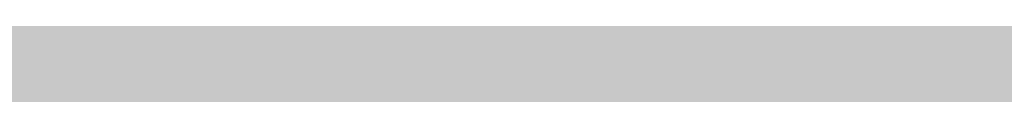
# Model space of a CAD drawing. Units: inches. Extents: x 2083 to 3317, y 1141 to 2115.
# Tile 153 of 256: x 3126.946713 to 3126.955939, y 1263.261932 to 1263.262504. Entities that reach past the tile are written whole.
import ezdxf

# ---------------------------------------------------------------- set-up
doc = ezdxf.new("R2010")
doc.units = ezdxf.units.IN
doc.layers.add('A-ANNO-DIMS', color=2, linetype='Continuous', lineweight=18)
doc.layers.add('A-WALL-PATT', color=251, linetype='Continuous', lineweight=13, true_color=0x636466)
doc.styles.get("Standard").update_dxf_attribs({"font": 'arial.ttf'})
doc.dimstyles.new('ISO-25', dxfattribs={"dimtxt": 12, "dimasz": 12, "dimexe": 1.25, "dimexo": 0.625, "dimtad": 1, "dimlunit": 3, "dimtxsty": 'Standard', "dimcen": 2.5, "dimadec": 0, "dimazin": 0, "dimtfac": 1, "dimtmove": 0, "dimatfit": 3, "dimfxl": 1, "dimarcsym": 0})

# ---------------------------------------------------------------- blocks, each defined once
blk = doc.blocks.new('*D26')
at = {"layer": 'A-ANNO-DIMS', "color": 0, "lineweight": -2, "transparency": 16777216}
for p, q in [((3088.985844, 1274.915092), (3088.985844, 1270.9519631)), ((3111.2400366, 1274.915092), (3111.2400366, 1270.9519631)), ((3076.985844, 1272.2019631), (2840.262447, 1272.2019631)), ((3111.2400366, 1272.2019631), (3088.985844, 1272.2019631)), ((3123.2400366, 1272.2019631), (3135.2400366, 1272.2019631))]:
    blk.add_line(p, q, dxfattribs=at)
at = {"layer": 'A-ANNO-DIMS', "color": 0, "transparency": 16777216}
for points in [[(3076.985844, 1274.2019631), (3076.985844, 1270.2019631), (3088.985844, 1272.2019631)], [(3123.2400366, 1274.2019631), (3123.2400366, 1270.2019631), (3111.2400366, 1272.2019631)]]:
    blk.add_solid(points, dxfattribs=at)
at = {"layer": 'Defpoints', "color": 0, "transparency": 16777216}
for p in [(3088.985844, 1275.540092), (3111.2400366, 1275.540092), (3088.985844, 1272.2019631)]:
    blk.add_point(p, dxfattribs=at)
at = {"layer": 'A-ANNO-DIMS', "color": 0, "transparency": 16777216, "insert": (2952.6241455, 1279.0316016), "char_height": 12, "attachment_point": 5}
blk.add_mtext('NIGHTSTAND 1\'-10 1/2" TYP.', dxfattribs=at)

msp = doc.modelspace()

# ---------------------------------------------------------------- hatches: boundary and pattern name
at = {"layer": 'A-WALL-PATT'}
h = msp.add_hatch(color=256, dxfattribs=at)
h.dxf.hatch_style = 1
h.paths.add_polyline_path([(3126.9597832, 2020.7613601), (2748.9597832, 2020.7613601), (2604.9597832, 2020.7613601), (2226.9597832, 2020.7613601), (2226.9597832, 1702.7613601), (2466.9597832, 1702.7613601), (2466.9597832, 1582.7613601), (2418.9597832, 1582.7613601), (2418.9597832, 1477.7613601), (2226.9597832, 1477.7613601), (2226.9597832, 1263.2613601), (2544.9597832, 1263.2613601), (2544.9597832, 1411.7613601), (2604.9597832, 1411.7613601), (2685.9597832, 1411.7613601), (2685.9597832, 1420.7613601), (2604.9597832, 1420.7613601), (2604.9597832, 1573.7613601), (2604.9597832, 1702.7613601), (2604.9597832, 2011.7613601), (2748.9597832, 2011.7613601), (2748.9597832, 1702.7613601), (2862.9597832, 1702.7613601), (2862.9597832, 1621.7613601), (2871.9597832, 1621.7613601), (2871.9597832, 1702.7613601), (2883.9597832, 1702.7613601), (2883.9597832, 1706.9394595, -0.026459), (2883.9597832, 1711.7613601), (2757.9597832, 1711.7613601), (2757.9597832, 1807.7613601), (2787.9597832, 1807.7613601), (2787.9597832, 1812.2613601), (2757.9597832, 1812.2613601), (2757.9597832, 2011.7613601), (2877.9597832, 2011.7613601), (2877.9597832, 1812.2613601), (2847.9597832, 1812.2613601), (2847.9597832, 1807.7613601), (2889.8357425, 1807.7613601), (2889.8357425, 1812.2613601), (2882.4597832, 1812.2613601), (2882.4597832, 2011.7613601), (3117.9597832, 2011.7613601), (3117.9597832, 1812.2613601), (2937.8357425, 1812.2613601), (2937.8357425, 1807.7613601), (2995.7097832, 1807.7613601), (2995.7097832, 1796.1176655), (3000.2097832, 1796.1176655), (3000.2097832, 1807.7613601), (3117.9597832, 1807.7613601), (3117.9597832, 1711.7613601), (3000.2097832, 1711.7613601), (3000.2097832, 1760.1176655), (2998.5727047, 1760.1176655, -0.020711), (2995.7097832, 1760.1176655), (2995.7097832, 1711.7613601), (2931.9597832, 1711.7613601), (2931.9597832, 1702.7613601), (3126.9597832, 1702.7613601)])
h.paths.add_polyline_path([(2471.4597832, 2011.7613601), (2471.4597832, 1810.0113601), (2462.7169357, 1810.0113601), (2462.7169357, 1805.5113601), (2505.9597832, 1805.5113601), (2505.9597832, 1810.0113601), (2475.9597832, 1810.0113601), (2475.9597832, 2011.7613601), (2595.9597832, 2011.7613601), (2595.9597832, 1810.0113601), (2565.9597832, 1810.0113601), (2565.9597832, 1805.5113601), (2595.9597832, 1805.5113601), (2595.9597832, 1711.7613601), (2235.9597832, 1711.7613601), (2235.9597832, 1805.5113601), (2353.7097832, 1805.5113601), (2353.7097832, 1796.0541624), (2358.2097832, 1796.0541624), (2358.2097832, 1805.5113601), (2414.7169357, 1805.5113601), (2414.7169357, 1810.0113601), (2235.9597832, 1810.0113601), (2235.9597832, 2011.7613601)], flags=16)
h.paths.add_polyline_path([(2270.2047343, 1994.6100082), (2270.2047343, 1970.6100082), (2246.2047343, 1970.6100082), (2246.2047343, 1994.6100082)], flags=0)
edge = h.paths.add_edge_path(flags=0)
edge.add_ellipse((2332.027391, 1899.7981761), major_axis=(-3.0429938, 3.0429938), ratio=0.16825245, start_angle=-161.3321656, end_angle=-156.3071136, ccw=False)
edge.add_ellipse((2333.0820373, 1898.7435297), major_axis=(-1.0546463, 1.0546463), ratio=0.453532097, start_angle=-123.371019, end_angle=-94.1591066)
edge = h.paths.add_edge_path(flags=0)
edge.add_ellipse((2332.027391, 1968.8762897), major_axis=(3.0429938, 3.0429938), ratio=0.16825245, start_angle=18.6678344, end_angle=23.6928864)
edge.add_spline(control_points=[(2332.9255964, 1970.6911045), (2332.2267681, 1970.3360997), (2330.8937087, 1969.6589054), (2328.4130803, 1970.9321376), (2327.2039345, 1967.7487119), (2324.7095965, 1969.9555886), (2322.5328223, 1967.012354), (2320.0128462, 1971.2958124), (2317.6803077, 1968.1578449), (2316.0405263, 1967.1020468), (2315.4269045, 1966.8096022)], knot_values=[0, 0, 0, 0, 2.267059, 4.324559, 6.685584, 8.878641, 11.121502, 14.300359, 17.755284, 19.732645, 19.732645, 19.732645, 19.732645], degree=3, periodic=0)
edge.add_ellipse((2332.027391, 1968.8762897), major_axis=(3.0429938, 3.0429938), ratio=0.16825245, start_angle=18.6678344, end_angle=23.6928864, ccw=False)
edge.add_ellipse((2333.0820373, 1969.930936), major_axis=(1.0546463, 1.0546463), ratio=0.453532097, start_angle=56.628981, end_angle=85.8408934, ccw=False)
edge = h.paths.add_edge_path(flags=0)
edge.add_spline(control_points=[(2296.4282874, 1967.9879081), (2293.6278045, 1965.3363137), (2287.7036238, 1959.727094), (2299.7438601, 1949.9956993), (2294.5325909, 1935.6685275), (2290.5732281, 1920.6035119), (2293.3941244, 1909.9736911), (2296.1854073, 1904.9665431)], knot_values=[0.099185, 0.099185, 0.099185, 0.099185, 0.345301, 0.619822, 0.982653, 1.386093, 1.810555, 1.810555, 1.810555, 1.810555], degree=3, periodic=0)
edge.add_spline(control_points=[(2296.1854073, 1904.9665431), (2297.3835817, 1902.6193002), (2298.0009694, 1901.9493116), (2298.5529698, 1901.4681549)], knot_values=[0.006246, 0.006246, 0.006246, 0.006246, 0.055476, 0.055476, 0.055476, 0.055476], degree=3, periodic=0)
edge.add_spline(control_points=[(2298.5529698, 1901.4681549), (2297.2586121, 1900.9232238), (2295.2252939, 1900.2321257), (2293.0602287, 1900.6142053), (2292.1014227, 1900.788415), (2292.0895776, 1900.790568)], knot_values=[0.312835, 0.312835, 0.312835, 0.312835, 0.40178, 0.474987, 0.475903, 0.475903, 0.475903, 0.475903], degree=3, periodic=0)
edge.add_arc((2292.7936464, 1904.6641088), 3.9370079, 215.4208969, 259.6981795, ccw=False)
edge.add_spline(control_points=[(2289.5853139, 1902.3823039), (2289.4766524, 1902.5350874), (2289.3684805, 1902.6880353), (2289.2608648, 1902.8411699)], knot_values=[0.102872, 0.102872, 0.102872, 0.102872, 0.116896, 0.116896, 0.116896, 0.116896], degree=3, periodic=0)
edge.add_spline(control_points=[(2289.2608648, 1902.8411699), (2288.6866042, 1902.5501922), (2287.6400477, 1902.0199025), (2285.8813368, 1901.8739536), (2283.8529717, 1901.5043521), (2281.7199871, 1899.7105375), (2278.4669913, 1899.492942), (2276.1571361, 1901.8832022), (2272.2589526, 1899.8040711), (2267.7776054, 1901.8431828), (2262.2438819, 1900.1840326), (2257.414927, 1901.7820606), (2254.318374, 1900.7261196), (2253.1782849, 1900.3373431)], knot_values=[0, 0, 0, 0, 1.907977, 3.477176, 5.261074, 7.972851, 11.680248, 13.717921, 16.939592, 22.789562, 27.502503, 33.595215, 37.145618, 37.145618, 37.145618, 37.145618], degree=3, periodic=0)
edge.add_line((2253.1782849, 1900.3373431), (2250.2442397, 1902.8411699))
edge.add_line((2250.2442397, 1902.8411699), (2250.2442397, 1965.8332959))
edge.add_line((2250.2442397, 1965.8332959), (2253.1782849, 1968.3371226))
edge.add_spline(control_points=[(2253.1782849, 1968.3371226), (2254.318374, 1967.9483462), (2257.414927, 1966.8924051), (2262.2438819, 1968.4904332), (2267.7776054, 1966.8312829), (2271.5267301, 1968.5372172), (2273.8759143, 1967.8282895), (2274.2067012, 1967.7276424)], knot_values=[0, 0, 0, 0, 0.09018, 0.244935, 0.364644, 0.513233, 0.537855, 0.537855, 0.537855, 0.537855], degree=3, periodic=0)
edge.add_arc((2274.3528869, 1963.7933495), 3.9370079, 72.0511336, 92.1279492, ccw=False)
edge.add_arc((2281.2969331, 1985.2300027), 18.5962982, 252.05113361, 288.56572166)
edge.add_arc((2292.3167172, 1956.0288805), 12.6460805, 71.02678788, 113.77821843, ccw=False)
edge = h.paths.add_edge_path(flags=0)
edge.add_spline(control_points=[(2274.8994147, 1951.8561946), (2275.066156, 1951.6165924), (2275.2326866, 1951.3765878), (2275.3979871, 1951.1358545)], knot_values=[1.409916, 1.409916, 1.409916, 1.409916, 1.43159, 1.43159, 1.43159, 1.43159], degree=3, periodic=0)
edge.add_spline(control_points=[(2275.3979871, 1951.1358545), (2275.7921055, 1950.5618854), (2276.1792311, 1949.9837745), (2276.5455462, 1949.3971029)], knot_values=[1.358238, 1.358238, 1.358238, 1.358238, 1.409916, 1.409916, 1.409916, 1.409916], degree=3, periodic=0)
edge.add_line((2276.5455462, 1949.3971029), (2277.437289, 1947.8621847))
edge.add_spline(control_points=[(2277.437289, 1947.8621847), (2276.3038341, 1945.6731147), (2274.6396979, 1942.4268817), (2274.631615, 1938.0938998), (2272.7991237, 1930.8515498), (2274.3564261, 1943.8970461), (2275.9476814, 1947.9233558), (2276.5455462, 1949.3971029)], knot_values=[0.005632, 0.005632, 0.005632, 0.005632, 0.186014, 0.266002, 0.357087, 0.59639, 0.739732, 0.739732, 0.739732, 0.739732], degree=3, periodic=0)
edge.add_spline(control_points=[(2276.5455462, 1949.3971029), (2276.1792311, 1949.9837745), (2275.7921055, 1950.5618854), (2275.3979871, 1951.1358545)], knot_values=[1.358238, 1.358238, 1.358238, 1.358238, 1.409916, 1.409916, 1.409916, 1.409916], degree=3, periodic=0)
edge.add_spline(control_points=[(2275.3979871, 1951.1358545), (2274.9425002, 1950.0804523), (2274.2077604, 1948.0252718), (2273.9346018, 1944.8514774), (2272.4685341, 1937.6274891), (2273.4662155, 1945.6964663), (2274.7006154, 1951.0594725), (2274.8994147, 1951.8561946)], knot_values=[0.104364, 0.104364, 0.104364, 0.104364, 0.189636, 0.269624, 0.36071, 0.600013, 0.644622, 0.644622, 0.644622, 0.644622], degree=3, periodic=0)
h.paths.add_polyline_path([(2269.1675139, 1963.1275729, -0.357527), (2268.170633, 1960.9763695, -0.092561), (2268.170633, 1939.4363249, -0.357527), (2269.1675139, 1937.2851215, -0.357527), (2267.0163105, 1938.2820024, -0.164785), (2254.6855813, 1938.2820024, -0.357527), (2252.5343779, 1937.2851215, -0.357527), (2253.5312587, 1939.4363249, -0.092561), (2253.5312587, 1960.9763695, -0.357527), (2252.5343779, 1963.1275729, -0.357527), (2254.6855813, 1962.130692, -0.164785), (2267.0163105, 1962.130692, -0.357527)], flags=0)
h.paths.add_polyline_path([(2248.8740679, 1967.8017998), (2248.8740679, 1957.0277095), (2249.4577833, 1957.0277095), (2249.4577833, 1911.6467562), (2248.8740679, 1911.6467562), (2248.8740679, 1900.8726659), (2246.5118632, 1900.8726659, 0.197327), (2244.1496584, 1902.4568734), (2244.1496584, 1966.2175923, 0.197327), (2246.5118632, 1967.8017998)], flags=0)
h.paths.add_polyline_path([(2269.1675139, 1931.3893442, -0.357527), (2268.170633, 1929.2381408, -0.092561), (2268.170633, 1907.6980962, -0.357527), (2269.1675139, 1905.5468928, -0.357527), (2267.0163105, 1906.5437737, -0.164785), (2254.6855813, 1906.5437737, -0.357527), (2252.5343779, 1905.5468928, -0.357527), (2253.5312587, 1907.6980962, -0.092561), (2253.5312587, 1929.2381408, -0.357527), (2252.5343779, 1931.3893442, -0.357527), (2254.6855813, 1930.3924634, -0.164785), (2267.0163105, 1930.3924634, -0.357527)], flags=0)
edge = h.paths.add_edge_path(flags=0)
edge.add_spline(control_points=[(2276.1968578, 1906.7237016), (2276.1681442, 1909.0289278), (2276.1140492, 1913.371852), (2270.5984171, 1924.9249783), (2273.9051746, 1919.0127787), (2275.9217115, 1916.2620626), (2275.4745699, 1912.4021495), (2277.2578735, 1910.3806206), (2276.6960436, 1908.2250358), (2276.6462176, 1906.8130226), (2276.6178249, 1906.0084068)], knot_values=[0, 0, 0, 0, 8.61026, 16.221274, 18.843057, 23.804898, 27.440828, 29.356102, 31.203478, 33.650687, 33.650687, 33.650687, 33.650687], degree=3, periodic=0)
edge.add_spline(control_points=[(2276.6178249, 1906.0084068), (2276.6233131, 1905.6241436), (2276.4977381, 1904.6286608), (2275.4417789, 1903.8547251), (2274.9373144, 1903.0804497), (2274.8590804, 1902.8411699)], knot_values=[0.156488, 0.156488, 0.156488, 0.156488, 0.184398, 0.231376, 0.250598, 0.250598, 0.250598, 0.250598], degree=3, periodic=0)
edge.add_line((2274.8590804, 1902.8411699), (2276.50598, 1902.8411699))
edge.add_spline(control_points=[(2276.50598, 1902.8411699), (2276.7883084, 1903.0849395), (2277.6650711, 1904.1251958), (2278.2495378, 1904.340738), (2277.6538719, 1908.5273866), (2278.15567, 1906.2278078), (2278.100464, 1905.2859484), (2278.8466748, 1904.0690054), (2277.8567853, 1903.4149482), (2277.8741909, 1902.9910497), (2277.9035616, 1902.8411699)], knot_values=[0.059574, 0.059574, 0.059574, 0.059574, 0.080753, 0.103741, 0.16972, 0.176036, 0.207137, 0.240474, 0.262341, 0.27366, 0.27366, 0.27366, 0.27366], degree=3, periodic=0)
edge.add_line((2277.9035616, 1902.8411699), (2280.0298255, 1902.8411699))
edge.add_spline(control_points=[(2280.0298255, 1902.8411699), (2279.8882214, 1903.088398), (2279.4992571, 1903.9815512), (2280.1522839, 1905.9393491), (2278.103615, 1909.6577572), (2279.7623946, 1907.185285), (2280.3279002, 1904.8748608), (2280.4851086, 1903.4895904), (2281.4632687, 1903.2494323), (2281.7583431, 1902.9364967), (2281.8340361, 1902.8411699)], knot_values=[0.013856, 0.013856, 0.013856, 0.013856, 0.034874, 0.088867, 0.107879, 0.126738, 0.158714, 0.193757, 0.217487, 0.226722, 0.226722, 0.226722, 0.226722], degree=3, periodic=0)
edge.add_spline(control_points=[(2281.8340361, 1902.8411699), (2281.7875348, 1902.8267029), (2281.6470224, 1902.7829881), (2281.3955272, 1902.85949), (2281.088077, 1902.9852418), (2280.7206826, 1903.060902), (2280.3334513, 1903.0257257), (2280.1247668, 1902.898879), (2280.0298255, 1902.8411699)], knot_values=[0, 0, 0, 0, 0.14413, 0.435517, 0.749276, 1.153046, 1.548371, 1.878348, 1.878348, 1.878348, 1.878348], degree=3, periodic=0)
edge.add_line((2280.0298255, 1902.8411699), (2277.9035616, 1902.8411699))
edge.add_spline(control_points=[(2277.9035616, 1902.8411699), (2277.892855, 1902.7958553), (2277.865396, 1902.6796374), (2277.6074793, 1902.6874828), (2277.2740503, 1902.8006999), (2276.8379209, 1902.6197745), (2276.5838074, 1902.7892611), (2276.50598, 1902.8411699)], knot_values=[0, 0, 0, 0, 0.127189, 0.326199, 0.628009, 1.24357, 1.515331, 1.515331, 1.515331, 1.515331], degree=3, periodic=0)
edge.add_line((2276.50598, 1902.8411699), (2274.8590804, 1902.8411699))
edge.add_spline(control_points=[(2274.8590804, 1902.8411699), (2274.8144367, 1902.8985868), (2274.7251297, 1903.013446), (2274.4934765, 1903.1189684), (2274.2442854, 1902.9605386), (2273.9371207, 1903.1849416), (2273.6140395, 1902.9831428), (2273.4083164, 1902.8830449), (2273.322254, 1902.8411699)], knot_values=[0, 0, 0, 0, 0.21843, 0.436957, 0.687977, 0.990379, 1.398396, 1.69185, 1.69185, 1.69185, 1.69185], degree=3, periodic=0)
edge.add_spline(control_points=[(2273.322254, 1902.8411699), (2273.6167403, 1903.445692), (2274.2739977, 1904.5382529), (2276.0272387, 1904.5737017), (2276.2069634, 1906.5836372), (2276.1968578, 1906.7237016)], knot_values=[0.012227, 0.012227, 0.012227, 0.012227, 0.059472, 0.106218, 0.134458, 0.134458, 0.134458, 0.134458], degree=3, periodic=0)
h.paths.add_polyline_path([(2270.7760538, 1897.7898284), (2270.7760538, 1873.7898284), (2246.7760538, 1873.7898284), (2246.7760538, 1897.7898284)], flags=0)
h.paths.add_polyline_path([(2353.7097832, 1760.0050593), (2353.7097832, 1760.0541624), (2358.2097832, 1760.0541624, -0.033729)], flags=0)
h.paths.add_polyline_path([(2321.8191188, 1737.5291862), (2341.9953271, 1737.5291862, -0.414214), (2343.2032727, 1736.3212406), (2343.2032727, 1721.0205964, -0.414214), (2341.9953271, 1719.8126508), (2321.8191188, 1719.8126508, -0.414214), (2320.6111732, 1721.0205964), (2320.6111732, 1736.3212406, -0.414214)], flags=0)
h.paths.add_polyline_path([(2324.2350099, 1736.3212406), (2339.5794359, 1736.3212406, -0.414214), (2341.9953271, 1733.9053494), (2341.9953271, 1725.4497302, -0.414214), (2339.5794359, 1723.033839), (2333.6805885, 1723.033839), (2333.8453172, 1722.0454666, -0.870646), (2335.4253988, 1721.8258934, -0.767327), (2333.922694, 1721.4232449), (2331.2910241, 1721.4232449, -0.767327), (2329.7883193, 1721.8258934, -0.870646), (2331.3684009, 1722.0454666), (2331.5331296, 1723.033839), (2324.2350099, 1723.033839, -0.414214), (2321.8191188, 1725.4497302), (2321.8191188, 1733.9053494, -0.414214)], flags=0)
h.paths.add_polyline_path([(2570.4837892, 1928.6154443), (2589.6837892, 1928.6154443), (2590.1688286, 1928.6154443), (2590.1688286, 1904.9933971), (2570.4837892, 1904.9933971)], flags=0)
h.paths.add_polyline_path([(2574.4473242, 1927.2638215, -1), (2572.8288357, 1927.2638215, -1)], flags=0)
h.paths.add_polyline_path([(2573.0898665, 1926.9408768), (2573.925032, 1927.7760423), (2574.1477428, 1927.5533315), (2573.3125773, 1926.718166)], flags=0)
h.paths.add_polyline_path([(2578.7790648, 1919.7296175, -1), (2571.5916632, 1919.7296175, -1)], flags=0)
h.paths.add_polyline_path([(2578.385364, 1919.7296175, -1), (2571.985364, 1919.7296175, -1)], flags=0)
h.paths.add_polyline_path([(2331.5957638, 1729.4762156, -1), (2333.6179542, 1729.4762156, -1)], flags=0)
h.paths.add_polyline_path([(2578.0342282, 1927.2638215, -1), (2576.4157396, 1927.2638215, -1)], flags=0)
h.paths.add_polyline_path([(2576.6888513, 1927.5310886), (2576.9115621, 1927.7537993), (2577.7467276, 1926.9186339), (2577.5240168, 1926.6959231)], flags=0)
h.paths.add_polyline_path([(2578.1390648, 1909.8595388, -1), (2572.2316632, 1909.8595388, -1)], flags=0)
h.paths.add_polyline_path([(2577.745364, 1909.8595388, -1), (2572.625364, 1909.8595388, -1)], flags=0)
h.paths.add_polyline_path([(2583.7977179, 1927.2638215, -1), (2582.1792294, 1927.2638215, -1)], flags=0)
h.paths.add_polyline_path([(2582.7186487, 1927.7537993), (2583.5538142, 1926.9186339), (2583.3311034, 1926.6959231), (2582.4959379, 1927.5310886)], flags=0)
h.paths.add_polyline_path([(2582.4959379, 1927.5310886), (2582.7186487, 1927.7537993), (2583.5538142, 1926.9186339), (2583.3311034, 1926.6959231)], flags=0)
h.paths.add_polyline_path([(2587.7390648, 1920.5296175, -1), (2581.8316632, 1920.5296175, -1)], flags=0)
h.paths.add_polyline_path([(2587.345364, 1920.5296175, -1), (2582.225364, 1920.5296175, -1)], flags=0)
h.paths.add_polyline_path([(2587.3846219, 1927.2638215, -1), (2585.7661333, 1927.2638215, -1)], flags=0)
h.paths.add_polyline_path([(2586.0819925, 1926.9802469), (2586.917158, 1927.8154124), (2587.1398688, 1927.5927016), (2586.3047033, 1926.7575361)], flags=0)
h.paths.add_polyline_path([(2588.3790648, 1910.6595388, -1), (2581.1916632, 1910.6595388, -1)], flags=0)
h.paths.add_polyline_path([(2587.985364, 1910.6595388, -1), (2581.585364, 1910.6595388, -1)], flags=0)
h.paths.add_polyline_path([(2417.1677288, 1729.4778955), (2437.3439372, 1729.4778955, -0.414214), (2438.5518828, 1728.2699499), (2438.5518828, 1712.9693057, -0.414214), (2437.3439372, 1711.7613601), (2417.1677288, 1711.7613601, -0.414214), (2415.9597832, 1712.9693057), (2415.9597832, 1728.2699499, -0.414214)], flags=0)
h.paths.add_polyline_path([(2419.58362, 1728.2699499), (2434.928046, 1728.2699499, -0.414214), (2437.3439372, 1725.8540587), (2437.3439372, 1717.3984395, -0.414214), (2434.928046, 1714.9825483), (2429.0291985, 1714.9825483), (2429.1939273, 1713.9941758, -0.870646), (2430.7740089, 1713.7746027, -0.767327), (2429.2713041, 1713.3719542), (2426.6396342, 1713.3719542, -0.767327), (2425.1369294, 1713.7746027, -0.870646), (2426.717011, 1713.9941758), (2426.8817397, 1714.9825483), (2419.58362, 1714.9825483, -0.414214), (2417.1677288, 1717.3984395), (2417.1677288, 1725.8540587, -0.414214)], flags=0)
h.paths.add_polyline_path([(2419.58362, 1728.2699499), (2434.928046, 1728.2699499, -0.414214), (2437.3439372, 1725.8540587), (2437.3439372, 1717.3984395, -0.414214), (2434.928046, 1714.9825483), (2429.0291985, 1714.9825483), (2428.3581177, 1719.0090337), (2427.5528206, 1719.0090337), (2426.8817397, 1714.9825483), (2419.58362, 1714.9825483, -0.414214), (2417.1677288, 1717.3984395), (2417.1677288, 1725.8540587, -0.414214)], flags=0)
h.paths.add_polyline_path([(2426.9443739, 1721.4249248, -1), (2428.9665643, 1721.4249248, -1)], flags=0)
h.paths.add_polyline_path([(2475.9597832, 1702.7613601), (2595.9597832, 1702.7613601), (2595.9597832, 1582.7613601), (2475.9597832, 1582.7613601)], flags=16)
h.paths.add_polyline_path([(2427.9597832, 1573.7613601), (2595.9597832, 1573.7613601), (2595.9597832, 1468.7613601), (2595.9597832, 1420.7613601), (2384.4597832, 1420.7613601), (2384.4597832, 1468.7613601), (2427.9597832, 1468.7613601)], flags=16)
h.paths.add_polyline_path([(2379.9597832, 1468.7613601), (2379.9597832, 1420.7613601), (2235.9597832, 1420.7613601), (2235.9597832, 1468.7613601)], flags=16)
h.paths.add_polyline_path([(2317.8159962, 1466.695767), (2337.9922045, 1466.695767, -0.414214), (2339.2001501, 1465.4878214), (2339.2001501, 1450.1871771, -0.414214), (2337.9922045, 1448.9792315), (2317.8159962, 1448.9792315, -0.414214), (2316.6080506, 1450.1871771), (2316.6080506, 1465.4878214, -0.414214)], flags=0)
h.paths.add_polyline_path([(2320.2318874, 1465.4878214), (2335.5763133, 1465.4878214, -0.414214), (2337.9922045, 1463.0719302), (2337.9922045, 1454.616311, -0.414214), (2335.5763133, 1452.2004198), (2329.6774659, 1452.2004198), (2329.8421946, 1451.2120473, -0.870646), (2331.4222762, 1450.9924742, -0.767327), (2329.9195714, 1450.5898257), (2327.2879015, 1450.5898257, -0.767327), (2325.7851967, 1450.9924742, -0.870646), (2327.3652783, 1451.2120473), (2327.530007, 1452.2004198), (2320.2318874, 1452.2004198, -0.414214), (2317.8159962, 1454.616311), (2317.8159962, 1463.0719302, -0.414214)], flags=0)
h.paths.add_polyline_path([(2320.2318874, 1465.4878214), (2335.5763133, 1465.4878214, -0.414214), (2337.9922045, 1463.0719302), (2337.9922045, 1454.616311, -0.414214), (2335.5763133, 1452.2004198), (2329.6774659, 1452.2004198), (2329.006385, 1456.2269051), (2328.2010879, 1456.2269051), (2327.530007, 1452.2004198), (2320.2318874, 1452.2004198, -0.414214), (2317.8159962, 1454.616311), (2317.8159962, 1463.0719302, -0.414214)], flags=0)
h.paths.add_polyline_path([(2327.5926413, 1458.6427963, -1), (2329.6148317, 1458.6427963, -1)], flags=0)
h.paths.add_polyline_path([(2244.4117436, 1433.3404531), (2241.9209449, 1433.3404531, -0.414214), (2240.0178562, 1435.2435418), (2240.0178562, 1440.9528078, -0.414211), (2241.920925, 1442.8558965), (2244.4117436, 1442.8558965, -1.976472)], flags=0)
h.paths.add_polyline_path([(2245.3568884, 1434.3975358, -0.414214), (2245.3568884, 1441.7988138, -2.144098)], flags=0)
h.paths.add_polyline_path([(2535.9597832, 1416.2613601), (2535.9597832, 1272.2613601), (2235.9597832, 1272.2613601), (2235.9597832, 1416.2613601)], flags=16)
h.paths.add_polyline_path([(2260.1195614, 1384.2928413), (2260.1195614, 1362.0386487), (2237.8653688, 1362.0386487), (2237.8653688, 1384.2928413)], flags=0)
edge = h.paths.add_edge_path(flags=0)
edge.add_line((2318.2518466, 1362.0932983), (2318.1457968, 1362.0009726))
edge.add_ellipse((2317.4451158, 1360.4310442), major_axis=(2.8216404, 2.8216404), ratio=0.16825245, start_angle=18.6678344, end_angle=20.9481273, ccw=False)
edge.add_ellipse((2318.4230451, 1361.4089735), major_axis=(0.9779293, 0.9779293), ratio=0.453532097, start_angle=56.628981, end_angle=70.2262012, ccw=False)
edge = h.paths.add_edge_path(flags=0)
edge.add_line((2319.1073699, 1295.5710784), (2319.0150442, 1295.6771282))
edge.add_ellipse((2317.4451158, 1296.3778091), major_axis=(-2.8216404, 2.8216404), ratio=0.16825245, start_angle=-161.3321656, end_angle=-159.0518727, ccw=False)
edge.add_ellipse((2318.4230451, 1295.3998798), major_axis=(-0.9779293, 0.9779293), ratio=0.453532097, start_angle=-123.371019, end_angle=-109.7737988)
edge = h.paths.add_edge_path(flags=0)
edge.add_spline(control_points=[(2284.2103489, 1301.1702189), (2284.5806878, 1300.444719), (2284.8911891, 1299.8920243), (2285.159553, 1299.4610182)], knot_values=[0.039066, 0.039066, 0.039066, 0.039066, 0.055476, 0.055476, 0.055476, 0.055476], degree=3, periodic=0)
edge.add_line((2285.159553, 1299.4610182), (2284.2103489, 1301.1702189))
edge = h.paths.add_edge_path(flags=0)
edge.add_line((2280.4124579, 1297.2980125), (2283.3699905, 1297.0361216))
edge.add_line((2283.3699905, 1297.0361216), (2286.4056902, 1297.9263104))
edge.add_spline(control_points=[(2286.4056902, 1297.9263104), (2285.305487, 1297.4631193), (2284.3447774, 1297.1291508), (2283.3699905, 1297.0361216)], knot_values=[0.394369, 0.394369, 0.394369, 0.394369, 0.475903, 0.475903, 0.475903, 0.475903], degree=3, periodic=0)
edge.add_spline(control_points=[(2283.3699905, 1297.0361216), (2283.2813895, 1297.027666), (2282.316289, 1296.9573356), (2281.3125019, 1297.1344787), (2280.4234414, 1297.2960161), (2280.4124579, 1297.2980125)], knot_values=[0.312835, 0.312835, 0.312835, 0.312835, 0.320246, 0.393453, 0.394369, 0.394369, 0.394369, 0.394369], degree=3, periodic=0)
edge = h.paths.add_edge_path(flags=0)
edge.add_line((2284.4355615, 1359.6072854), (2280.4462909, 1355.328047))
edge.add_line((2280.4462909, 1355.328047), (2279.5799868, 1351.0177544))
edge.add_line((2279.5799868, 1351.0177544), (2282.4129737, 1346.5804327))
edge.add_spline(control_points=[(2282.4129737, 1346.5804327), (2283.1533308, 1345.5892358), (2284.2528957, 1344.0288973), (2284.801037, 1342.3871671), (2284.9351625, 1341.8055443)], knot_values=[1.240098, 1.240098, 1.240098, 1.240098, 1.332892, 1.382712, 1.382712, 1.382712, 1.382712], degree=3, periodic=0)
edge.add_spline(control_points=[(2284.9351625, 1341.8055443), (2285.3191079, 1340.1406002), (2285.2330291, 1338.4092041), (2284.9099384, 1336.6541222)], knot_values=[1.097484, 1.097484, 1.097484, 1.097484, 1.240098, 1.240098, 1.240098, 1.240098], degree=3, periodic=0)
edge.add_spline(control_points=[(2284.9099384, 1336.6541222), (2284.5868478, 1334.8990403), (2284.0267453, 1333.1202725), (2283.4626437, 1331.3605849)], knot_values=[0.95487, 0.95487, 0.95487, 0.95487, 1.097484, 1.097484, 1.097484, 1.097484], degree=3, periodic=0)
edge.add_line((2283.4626437, 1331.3605849), (2281.8903759, 1326.153357))
edge.add_line((2281.8903759, 1326.153357), (2280.7562592, 1321.0560888))
edge.add_line((2280.7562592, 1321.0560888), (2280.2992048, 1316.0019772))
edge.add_line((2280.2992048, 1316.0019772), (2280.7159327, 1310.9500678))
edge.add_line((2280.7159327, 1310.9500678), (2282.0280939, 1305.9721367))
edge.add_line((2282.0280939, 1305.9721367), (2284.2103489, 1301.1702189))
edge.add_spline(control_points=[(2284.2103489, 1301.1702189), (2283.3407305, 1302.7301854), (2282.6119044, 1304.3364933), (2282.0280939, 1305.9721367)], knot_values=[0.099185, 0.099185, 0.099185, 0.099185, 0.241799, 0.241799, 0.241799, 0.241799], degree=3, periodic=0)
edge.add_spline(control_points=[(2282.0280939, 1305.9721367), (2281.4442835, 1307.6077801), (2281.0054886, 1309.2727591), (2280.7159327, 1310.9500678)], knot_values=[0.241799, 0.241799, 0.241799, 0.241799, 0.384413, 0.384413, 0.384413, 0.384413], degree=3, periodic=0)
edge.add_spline(control_points=[(2280.7159327, 1310.9500678), (2280.4332411, 1312.5876134), (2280.2893863, 1314.2769594), (2280.2988938, 1315.9620324), (2280.2992048, 1316.0019772)], knot_values=[0.384413, 0.384413, 0.384413, 0.384413, 0.523647, 0.527028, 0.527028, 0.527028, 0.527028], degree=3, periodic=0)
edge.add_spline(control_points=[(2280.2992048, 1316.0019772), (2280.3123257, 1317.6869552), (2280.4778706, 1319.3679256), (2280.7562592, 1321.0560888)], knot_values=[0.527028, 0.527028, 0.527028, 0.527028, 0.669642, 0.669642, 0.669642, 0.669642], degree=3, periodic=0)
edge.add_spline(control_points=[(2280.7562592, 1321.0560888), (2281.0346478, 1322.7442519), (2281.4258801, 1324.4396079), (2281.8903759, 1326.153357)], knot_values=[0.669642, 0.669642, 0.669642, 0.669642, 0.812256, 0.812256, 0.812256, 0.812256], degree=3, periodic=0)
edge.add_spline(control_points=[(2281.8903759, 1326.153357), (2282.2643834, 1327.5332507), (2282.7878702, 1329.2618097), (2283.352751, 1331.0177803), (2283.4626437, 1331.3605849)], knot_values=[0.812256, 0.812256, 0.812256, 0.812256, 0.927087, 0.95487, 0.95487, 0.95487, 0.95487], degree=3, periodic=0)
edge.add_line((2283.4626437, 1331.3605849), (2284.9099384, 1336.6541222))
edge.add_line((2284.9099384, 1336.6541222), (2284.9351625, 1341.8055443))
edge.add_line((2284.9351625, 1341.8055443), (2282.4129737, 1346.5804327))
edge.add_spline(control_points=[(2282.4129737, 1346.5804327), (2281.2751273, 1348.1037918), (2280.0784467, 1349.5703178), (2279.5799868, 1351.0177544)], knot_values=[1.382712, 1.382712, 1.382712, 1.382712, 1.525326, 1.525326, 1.525326, 1.525326], degree=3, periodic=0)
edge.add_spline(control_points=[(2279.5799868, 1351.0177544), (2279.4432818, 1351.4147209), (2279.1363124, 1352.856922), (2279.7351897, 1354.2903851), (2280.4462909, 1355.328047)], knot_values=[1.525326, 1.525326, 1.525326, 1.525326, 1.564439, 1.667941, 1.667941, 1.667941, 1.667941], degree=3, periodic=0)
edge.add_spline(control_points=[(2280.4462909, 1355.328047), (2281.4261132, 1356.7578354), (2282.9308373, 1358.1825604), (2284.4355615, 1359.6072854)], knot_values=[1.667941, 1.667941, 1.667941, 1.667941, 1.810555, 1.810555, 1.810555, 1.810555], degree=3, periodic=0)
edge.add_arc((2280.6230749, 1348.518181), 11.7261796, 71.02678788, 113.77821843)
edge.add_arc((2270.4048917, 1375.5951559), 17.2435667, 252.05113361, 288.56572166, ccw=False)
edge.add_arc((2263.9659692, 1355.7178471), 3.6506221, 72.0511336, 92.1279492)
edge.add_arc((2263.9659692, 1355.7178471), 3.6506221, 92.1279492, 177.98513)
edge.add_spline(control_points=[(2260.3176041, 1355.8461989), (2260.2604169, 1354.2206683), (2260.551278, 1350.1865469), (2262.9993445, 1346.7662507), (2264.4727415, 1344.6490245)], knot_values=[1.43159, 1.43159, 1.43159, 1.43159, 1.564144, 1.770695, 1.770695, 1.770695, 1.770695], degree=3, periodic=0)
edge.add_line((2264.4727415, 1344.6490245), (2264.9355904, 1343.9825301))
edge.add_spline(control_points=[(2263.8010444, 1340.2481052), (2263.8432379, 1340.5140884), (2264.0672444, 1341.7564652), (2264.5126928, 1343.0024532), (2264.9350468, 1343.9810834)], knot_values=[0.53657, 0.53657, 0.53657, 0.53657, 0.559349, 0.644622, 0.644622, 0.644622, 0.644622], degree=3, periodic=0)
edge.add_spline(control_points=[(2264.9350468, 1343.9810834), (2265.1177715, 1343.7149747), (2265.2988751, 1343.4479058), (2265.4767562, 1343.1793646)], knot_values=[1.384077, 1.384077, 1.384077, 1.384077, 1.409916, 1.409916, 1.409916, 1.409916], degree=3, periodic=0)
edge.add_spline(control_points=[(2265.4767562, 1343.1793646), (2265.6546373, 1342.9108234), (2265.8292958, 1342.64081), (2265.9991301, 1342.368812)], knot_values=[1.358238, 1.358238, 1.358238, 1.358238, 1.384077, 1.384077, 1.384077, 1.384077], degree=3, periodic=0)
edge.add_line((2265.9991301, 1342.368812), (2266.8260057, 1340.9455468))
edge.add_spline(control_points=[(2266.8260057, 1340.9455468), (2268.894401, 1337.0896912), (2271.3981727, 1325.8430009), (2270.5161644, 1310.5685568), (2275.9193759, 1301.860609), (2277.7895113, 1299.1994495)], knot_values=[0.116896, 0.116896, 0.116896, 0.116896, 0.472987, 1.050969, 1.313793, 1.313793, 1.313793, 1.313793], degree=3, periodic=0)
edge.add_spline(control_points=[(2277.7895113, 1299.1994495), (2277.8394051, 1299.1284519), (2277.8894277, 1299.0574975), (2277.9395717, 1298.9865839)], knot_values=[0.109884, 0.109884, 0.109884, 0.109884, 0.116896, 0.116896, 0.116896, 0.116896], degree=3, periodic=0)
edge.add_line((2277.9395717, 1298.9865839), (2277.7888489, 1299.1991139))
edge.add_spline(control_points=[(2277.7888489, 1299.1991139), (2277.2565819, 1298.9294144), (2276.2863504, 1298.4379024), (2275.0393517, 1298.3344186), (2274.3833299, 1298.2388951), (2274.2152543, 1298.209338)], knot_values=[33.12187, 33.12187, 33.12187, 33.12187, 35.029056, 36.598255, 37.144827, 37.144827, 37.144827, 37.144827], degree=3, periodic=0)
edge.add_line((2274.2152543, 1298.209338), (2273.073147, 1297.8929607))
edge.add_spline(control_points=[(2273.073147, 1297.8929607), (2272.3229363, 1297.579784), (2271.0391507, 1296.5105078), (2269.2483948, 1296.2260622), (2268.4231004, 1296.3746543)], knot_values=[26.532584, 26.532584, 26.532584, 26.532584, 29.198919, 31.839101, 31.839101, 31.839101, 31.839101], degree=3, periodic=0)
edge.add_line((2268.4231004, 1296.3746543), (2263.8785014, 1297.4575338))
edge.add_spline(control_points=[(2263.8785014, 1297.4575338), (2263.5560769, 1297.3594345), (2261.8603064, 1296.8386943), (2260.2387805, 1297.2824073), (2258.9334543, 1297.5164611)], knot_values=[15.919551, 15.919551, 15.919551, 15.919551, 16.939592, 21.226067, 21.226067, 21.226067, 21.226067], degree=3, periodic=0)
edge.add_line((2258.9334543, 1297.5164611), (2254.0552332, 1297.3290098))
edge.add_spline(control_points=[(2254.0552332, 1297.3290098), (2253.7555255, 1297.295815), (2252.1136834, 1297.1651738), (2250.4618687, 1297.5442209), (2249.1296862, 1297.6678818)], knot_values=[5.306517, 5.306517, 5.306517, 5.306517, 6.276435, 10.613034, 10.613034, 10.613034, 10.613034], degree=3, periodic=0)
edge.add_line((2249.1296862, 1297.6678818), (2244.3316495, 1296.8777561))
edge.add_line((2244.3316495, 1296.8777561), (2241.6110326, 1299.1994495))
edge.add_line((2241.6110326, 1299.1994495), (2241.6110326, 1357.6094038))
edge.add_line((2241.6110326, 1357.6094038), (2244.3316495, 1359.9310973))
edge.add_line((2244.3316495, 1359.9310973), (2252.7288228, 1359.5426917))
edge.add_spline(control_points=[(2252.7288228, 1359.5426917), (2252.8709387, 1359.5464396), (2253.3057402, 1359.5481716), (2253.7398447, 1359.5142744), (2254.0317419, 1359.4824261)], knot_values=[0.233291, 0.233291, 0.233291, 0.233291, 0.244935, 0.268927, 0.268927, 0.268927, 0.268927], degree=3, periodic=0)
edge.add_line((2254.0317419, 1359.4824261), (2259.5871899, 1359.4163899))
edge.add_spline(control_points=[(2259.5871899, 1359.4163899), (2260.6770676, 1359.6285026), (2262.0731971, 1359.8970025), (2263.5236925, 1359.4592776), (2263.8304173, 1359.3659518)], knot_values=[0.422516, 0.422516, 0.422516, 0.422516, 0.513233, 0.537855, 0.537855, 0.537855, 0.537855], degree=3, periodic=0)
edge.add_arc((2263.9659692, 1355.7178471), 3.6506221, 72.0511336, 92.1279492, ccw=False)
edge.add_arc((2270.4048917, 1375.5951559), 17.2435667, 252.05113361, 288.56572166)
edge.add_arc((2280.6230749, 1348.518181), 11.7261796, 71.02678788, 113.77821843, ccw=False)
h.paths.add_polyline_path([(2240.3405298, 1359.4347149), (2240.3405298, 1349.4443532), (2240.8817846, 1349.4443532), (2240.8817846, 1307.3645001), (2240.3405298, 1307.3645001), (2240.3405298, 1297.3741385), (2238.1501565, 1297.3741385, 0.197327), (2235.9597832, 1298.8431076), (2235.9597832, 1357.9657458, 0.197327), (2238.1501565, 1359.4347149)], flags=0)
h.paths.add_polyline_path([(2259.1577904, 1355.1005005, -0.357527), (2258.2334246, 1353.1057799, -0.092561), (2258.2334246, 1333.1326007, -0.357527), (2259.1577904, 1331.1378801, -0.357527), (2257.1630698, 1332.0622458, -0.164785), (2245.7293022, 1332.0622458, -0.357527), (2243.7345816, 1331.1378801, -0.357527), (2244.6589474, 1333.1326007, -0.092561), (2244.6589474, 1353.1057799, -0.357527), (2243.7345816, 1355.1005005, -0.357527), (2245.7293022, 1354.1761347, -0.164785), (2257.1630698, 1354.1761347, -0.357527)], flags=0)
edge = h.paths.add_edge_path(flags=0)
edge.add_line((2265.9991301, 1342.368812), (2266.8260057, 1340.9455468))
edge.add_line((2266.8260057, 1340.9455468), (2265.3075567, 1337.8140664))
edge.add_line((2265.3075567, 1337.8140664), (2264.358232, 1334.6529388))
edge.add_line((2264.358232, 1334.6529388), (2264.2620123, 1333.7997046))
edge.add_spline(control_points=[(2264.2620123, 1333.7997046), (2264.2083565, 1333.187055), (2264.1620602, 1332.3655252), (2264.0071444, 1331.4139326), (2263.9690487, 1331.2018338)], knot_values=[0.464444, 0.464444, 0.464444, 0.464444, 0.516691, 0.531608, 0.531608, 0.531608, 0.531608], degree=3, periodic=0)
edge.add_spline(control_points=[(2263.9690487, 1331.2018338), (2263.7745349, 1330.1188727), (2263.4243703, 1328.7908386), (2263.2574202, 1328.5306516), (2263.2340282, 1328.5146115)], knot_values=[0.372682, 0.372682, 0.372682, 0.372682, 0.44885, 0.464444, 0.464444, 0.464444, 0.464444], degree=3, periodic=0)
edge.add_spline(control_points=[(2263.2340282, 1328.5146115), (2263.096382, 1328.4202271), (2263.1311696, 1329.3014765), (2263.2749528, 1330.6157493)], knot_values=[0.280919, 0.280919, 0.280919, 0.280919, 0.372682, 0.372682, 0.372682, 0.372682], degree=3, periodic=0)
edge.add_spline(control_points=[(2263.2749528, 1330.6157493), (2263.4187361, 1331.930022), (2263.6715151, 1333.677318), (2263.9698519, 1335.3150268)], knot_values=[0.189157, 0.189157, 0.189157, 0.189157, 0.280919, 0.280919, 0.280919, 0.280919], degree=3, periodic=0)
edge.add_spline(control_points=[(2263.9698519, 1335.3150268), (2264.1004958, 1336.0321917), (2264.4187827, 1337.6219113), (2264.7548476, 1338.8644304), (2264.9474193, 1339.4911244)], knot_values=[0.097394, 0.097394, 0.097394, 0.097394, 0.137578, 0.189157, 0.189157, 0.189157, 0.189157], degree=3, periodic=0)
edge.add_spline(control_points=[(2264.9474193, 1339.4911244), (2265.2900171, 1340.6060546), (2265.6442376, 1341.4939958), (2265.9991301, 1342.368812)], knot_values=[0.005632, 0.005632, 0.005632, 0.005632, 0.097394, 0.097394, 0.097394, 0.097394], degree=3, periodic=0)
h.paths.add_polyline_path([(2259.1577904, 1325.6709733, -0.357527), (2258.2334246, 1323.6762527, -0.092561), (2258.2334246, 1303.7030735, -0.357527), (2259.1577904, 1301.7083529, -0.357527), (2257.1630698, 1302.6327186, -0.164785), (2245.7293022, 1302.6327186, -0.357527), (2243.7345816, 1301.7083529, -0.357527), (2244.6589474, 1303.7030735, -0.092561), (2244.6589474, 1323.6762527, -0.357527), (2243.7345816, 1325.6709733, -0.357527), (2245.7293022, 1324.7466075, -0.164785), (2257.1630698, 1324.7466075, -0.357527)], flags=0)
edge = h.paths.add_edge_path(flags=0)
edge.add_spline(control_points=[(2261.7089377, 1317.3114208), (2261.6794818, 1317.4175798), (2261.7618581, 1317.3885347), (2262.4907358, 1316.0898725), (2262.962185, 1315.3008975)], knot_values=[14.955861, 14.955861, 14.955861, 14.955861, 16.221274, 18.694826, 18.694826, 18.694826, 18.694826], degree=3, periodic=0)
edge.add_spline(control_points=[(2262.962185, 1315.3008975), (2262.9904374, 1315.2536169), (2263.7020958, 1314.0673762), (2264.3489834, 1313.1271533), (2264.7300545, 1312.1641544)], knot_values=[18.694826, 18.694826, 18.694826, 18.694826, 18.843057, 22.433791, 22.433791, 22.433791, 22.433791], degree=3, periodic=0)
edge.add_spline(control_points=[(2264.7300545, 1312.1641544), (2264.8755649, 1311.7964373), (2265.1768733, 1310.7698073), (2265.1430689, 1309.5592623), (2265.2477363, 1308.8241926)], knot_values=[22.433791, 22.433791, 22.433791, 22.433791, 23.804898, 26.172756, 26.172756, 26.172756, 26.172756], degree=3, periodic=0)
edge.add_line((2265.2477363, 1308.8241926), (2265.8507741, 1307.1718879))
edge.add_spline(control_points=[(2265.8507741, 1307.1718879), (2266.0650246, 1306.8216779), (2266.3843872, 1306.3322461), (2266.4244001, 1305.7805489), (2266.4203688, 1305.6112163)], knot_values=[28.062562, 28.062562, 28.062562, 28.062562, 29.356102, 29.911721, 29.911721, 29.911721, 29.911721], degree=3, periodic=0)
edge.add_spline(control_points=[(2266.4203688, 1305.6112163), (2266.4161162, 1305.4325896), (2266.393999, 1305.2499979), (2266.3647773, 1305.0658571)], knot_values=[29.911721, 29.911721, 29.911721, 29.911721, 30.497837, 30.497837, 30.497837, 30.497837], degree=3, periodic=0)
edge.add_line((2266.3647773, 1305.0658571), (2266.0661511, 1302.1362954))
edge.add_spline(control_points=[(2266.0661511, 1302.1362954), (2266.0712401, 1301.7799843), (2265.9980761, 1301.1999847), (2265.6632664, 1300.7589613), (2265.5089084, 1300.5858824)], knot_values=[0.156488, 0.156488, 0.156488, 0.156488, 0.184398, 0.203543, 0.203543, 0.203543, 0.203543], degree=3, periodic=0)
edge.add_line((2265.5089084, 1300.5858824), (2264.4353411, 1299.1994495))
edge.add_line((2264.4353411, 1299.1994495), (2265.962442, 1299.1994495))
edge.add_line((2265.962442, 1299.1994495), (2267.3359898, 1301.1752758))
edge.add_line((2267.3359898, 1301.1752758), (2267.3116668, 1301.9862366))
edge.add_spline(control_points=[(2267.3116668, 1301.9862366), (2267.261111, 1302.8623959), (2267.1602121, 1303.7371316), (2267.2714865, 1303.3258962)], knot_values=[0.126229, 0.126229, 0.126229, 0.126229, 0.166617, 0.166617, 0.166617, 0.166617], degree=3, periodic=0)
edge.add_spline(control_points=[(2267.2714865, 1303.3258962), (2267.2800347, 1303.2943047), (2267.3097851, 1303.1753659), (2267.3734504, 1302.8836084), (2267.4061233, 1302.6828291), (2267.4179259, 1302.6010251)], knot_values=[0.166617, 0.166617, 0.166617, 0.166617, 0.16972, 0.176036, 0.180765, 0.180765, 0.180765, 0.180765], degree=3, periodic=0)
edge.add_spline(control_points=[(2267.7438914, 1300.9875045), (2267.6875832, 1301.1509426), (2267.4805198, 1301.6566644), (2267.4837514, 1302.1447877), (2267.4179259, 1302.6010251)], knot_values=[0.180765, 0.180765, 0.180765, 0.180765, 0.193767, 0.220139, 0.220139, 0.220139, 0.220139], degree=3, periodic=0)
edge.add_line((2267.4179259, 1302.6010251), (2267.7438914, 1300.9875045))
edge.add_spline(control_points=[(2267.7438914, 1300.9875045), (2267.8319608, 1300.7318778), (2267.9320205, 1300.3099042), (2267.5548409, 1299.9745185), (2267.429366, 1299.8292073)], knot_values=[0.220139, 0.220139, 0.220139, 0.220139, 0.240474, 0.25489, 0.25489, 0.25489, 0.25489], degree=3, periodic=0)
edge.add_line((2267.429366, 1299.8292073), (2267.2583608, 1299.1994495))
edge.add_line((2267.2583608, 1299.1994495), (2269.229956, 1299.1994495))
edge.add_spline(control_points=[(2269.229956, 1299.1994495), (2269.0986525, 1299.4286938), (2268.842774, 1300.0162509), (2269.0115749, 1300.9159235), (2268.9467957, 1301.6607397)], knot_values=[0.013856, 0.013856, 0.013856, 0.013856, 0.034874, 0.067073, 0.067073, 0.067073, 0.067073], degree=3, periodic=0)
edge.add_line((2268.9467957, 1301.6607397), (2268.4315815, 1303.6031089))
edge.add_spline(control_points=[(2268.4315815, 1303.6031089), (2268.1755957, 1304.1923747), (2267.5962136, 1305.2512977), (2268.0406981, 1304.6232098), (2268.2513938, 1304.2824205)], knot_values=[0.090155, 0.090155, 0.090155, 0.090155, 0.107879, 0.120289, 0.120289, 0.120289, 0.120289], degree=3, periodic=0)
edge.add_spline(control_points=[(2268.2513938, 1304.2824205), (2268.3608818, 1304.1053294), (2269.0577527, 1302.9179833), (2269.382691, 1301.5904186), (2269.5214051, 1300.7759312), (2269.5752202, 1300.5557836)], knot_values=[0.120289, 0.120289, 0.120289, 0.120289, 0.126738, 0.158714, 0.173506, 0.173506, 0.173506, 0.173506], degree=3, periodic=0)
edge.add_line((2269.5752202, 1300.5557836), (2270.6857984, 1299.4212579))
edge.add_spline(control_points=[(2270.6857984, 1299.4212579), (2270.7672206, 1299.3572512), (2270.8378523, 1299.2814011), (2270.9029248, 1299.1994495)], knot_values=[0.21816, 0.21816, 0.21816, 0.21816, 0.226722, 0.226722, 0.226722, 0.226722], degree=3, periodic=0)
edge.add_line((2270.9372012, 1299.1929131), (2270.9029248, 1299.1994495))
edge.add_spline(control_points=[(2270.9029248, 1299.1994495), (2270.8598061, 1299.1860349), (2270.7295148, 1299.1455), (2270.4963139, 1299.216437), (2270.2716612, 1299.3083234), (2270.1210168, 1299.3479612), (2270.0633386, 1299.3595566)], knot_values=[0.939174, 0.939174, 0.939174, 0.939174, 1.083304, 1.374691, 1.68845, 1.878348, 1.878348, 1.878348, 1.878348], degree=3, periodic=0)
edge.add_line((2270.0633386, 1299.3595566), (2269.229956, 1299.1994495))
edge.add_line((2269.229956, 1299.1994495), (2267.2583608, 1299.1994495))
edge.add_spline(control_points=[(2267.2583608, 1299.1994495), (2267.248433, 1299.1574312), (2267.2229714, 1299.0496673), (2266.9838161, 1299.056942), (2266.8092097, 1299.1162303), (2266.6769047, 1299.1090913), (2266.636531, 1299.1048147)], knot_values=[0.757665, 0.757665, 0.757665, 0.757665, 0.884854, 1.083864, 1.385675, 1.515331, 1.515331, 1.515331, 1.515331], degree=3, periodic=0)
edge.add_spline(control_points=[(2266.636531, 1299.1048147), (2266.4852248, 1299.0887878), (2266.2358066, 1299.0171229), (2266.0346081, 1299.1513168), (2265.962442, 1299.1994495)], knot_values=[0, 0, 0, 0, 0.485905, 0.757665, 0.757665, 0.757665, 0.757665], degree=3, periodic=0)
edge.add_line((2265.962442, 1299.1994495), (2264.4353411, 1299.1994495))
edge.add_line((2264.4353411, 1299.1994495), (2263.8584442, 1299.3671176))
edge.add_spline(control_points=[(2263.8584442, 1299.3671176), (2263.8189433, 1299.3709053), (2263.7795277, 1299.3857212), (2263.7401308, 1299.4015039)], knot_values=[0.845925, 0.845925, 0.845925, 0.845925, 0.978627, 0.978627, 0.978627, 0.978627], degree=3, periodic=0)
edge.add_line((2263.7217862, 1299.3964251), (2263.0103065, 1299.1994495))
edge.add_spline(control_points=[(2263.0103065, 1299.1994495), (2263.2457942, 1299.682859), (2263.5060317, 1300.1281072), (2263.8734943, 1300.4080279)], knot_values=[0.012227, 0.012227, 0.012227, 0.012227, 0.052971, 0.052971, 0.052971, 0.052971], degree=3, periodic=0)
edge.add_spline(control_points=[(2263.8734943, 1300.4080279), (2263.932131, 1300.4526954), (2264.0842429, 1300.5529789), (2264.2551889, 1300.6242227), (2264.3596855, 1300.6647475)], knot_values=[0.052971, 0.052971, 0.052971, 0.052971, 0.059472, 0.069086, 0.069086, 0.069086, 0.069086], degree=3, periodic=0)
edge.add_line((2264.3596855, 1300.6647475), (2265.1418998, 1301.0777737))
edge.add_line((2265.1418998, 1301.0777737), (2265.675806, 1302.7995583))
edge.add_line((2265.675806, 1302.7995583), (2265.5407004, 1305.7040662))
edge.add_line((2265.5407004, 1305.7040662), (2264.8030733, 1309.3277237))
edge.add_line((2264.8030733, 1309.3277237), (2263.0405349, 1314.0917906))
edge.add_spline(control_points=[(2263.0405349, 1314.0917906), (2262.3835724, 1315.6714379), (2261.7959724, 1316.9977489), (2261.7089377, 1317.3114208)], knot_values=[11.216896, 11.216896, 11.216896, 11.216896, 14.955861, 14.955861, 14.955861, 14.955861], degree=3, periodic=0)
h.paths.add_polyline_path([(2871.9597832, 1416.2613601), (2895.910047, 1416.2613601), (2895.910047, 1420.7613601), (2871.9597832, 1420.7613601), (2871.9597832, 1501.7613601), (2862.9597832, 1501.7613601), (2862.9597832, 1420.7613601), (2805.9597832, 1420.7613601), (2805.9597832, 1411.7613601), (2862.9597832, 1411.7613601), (2862.9597832, 1263.2613601), (3126.9597832, 1263.2613601), (3126.9597832, 1411.7613601), (3126.9597832, 1486.7613601), (2943.9597832, 1486.7613601), (2943.9597832, 1477.7613601), (2967.8603109, 1477.7613601), (2967.8603109, 1420.7613601), (2943.910047, 1420.7613601), (2943.910047, 1416.2613601), (3117.9597832, 1416.2613601), (3117.9597832, 1420.7613601), (2972.3603109, 1420.7613601), (2972.3603109, 1477.7613601), (3117.9597832, 1477.7613601), (3117.9597832, 1420.7613601), (3117.9597832, 1272.2613601), (2871.9597832, 1272.2613601)], flags=0)
h.paths.add_polyline_path([(2457.1256256, 1485.9425054), (2527.6026508, 1485.9425054), (2527.6026508, 1537.6357021), (2457.1256256, 1537.6357021)], flags=8)
h.paths.add_polyline_path([(2481.0050583, 1609.9818039), (2590.765818, 1609.9818039), (2590.765818, 1682.0033623), (2481.0050583, 1682.0033623)], flags=8)
h.paths.add_polyline_path([(2483.0850224, 1729.1267835), (2553.5620476, 1729.1267835), (2553.5620476, 1780.8199802), (2483.0850224, 1780.8199802)], flags=8)
h = msp.add_hatch(color=256, dxfattribs=at)
h.dxf.hatch_style = 1
h.paths.add_polyline_path([(3126.9597832, 1486.7613601), (2943.9597832, 1486.7613601), (2943.9597832, 1477.7613601), (2967.8603109, 1477.7613601), (2967.8603109, 1420.7613601), (2943.910047, 1420.7613601), (2943.910047, 1416.2613601), (3117.9597832, 1416.2613601), (3117.9597832, 1420.7613601), (2972.3603109, 1420.7613601), (2972.3603109, 1477.7613601), (3117.9597832, 1477.7613601), (3117.9597832, 1420.7613601), (3117.9597832, 1272.2613601), (2871.9597832, 1272.2613601), (2871.9597832, 1416.2613601), (2895.910047, 1416.2613601), (2895.910047, 1420.7613601), (2871.9597832, 1420.7613601), (2871.9597832, 1501.7613601), (2862.9597832, 1501.7613601), (2862.9597832, 1420.7613601), (2805.9597832, 1420.7613601), (2805.9597832, 1411.7613601), (2862.9597832, 1411.7613601), (2862.9597832, 1263.2613601), (3126.9597832, 1263.2613601), (3126.9597832, 1411.7613601)])

# ---------------------------------------------------------------- dimensions: what is measured, and where the dimension line sits
at = {"layer": 'A-ANNO-DIMS'}
dim = msp.add_linear_dim(base=(3088.985844, 1272.2019631), p1=(3111.2400366, 1275.540092), p2=(3088.985844, 1275.540092), angle=180, text='NIGHTSTAND <> TYP.', dimstyle='ISO-25', override={"dimdec": 1, "dimlfac": 1, "dimrnd": 0, "dimzin": 1, "dimdsep": 46, "dimlunit": 4, "dimfrac": 2}, dxfattribs=at)
dim.commit()
dim.dimension.update_dxf_attribs({"geometry": '*D26', "text_midpoint": (2952.6241455, 1279.0316016)})

doc.saveas('drawing.dxf')
